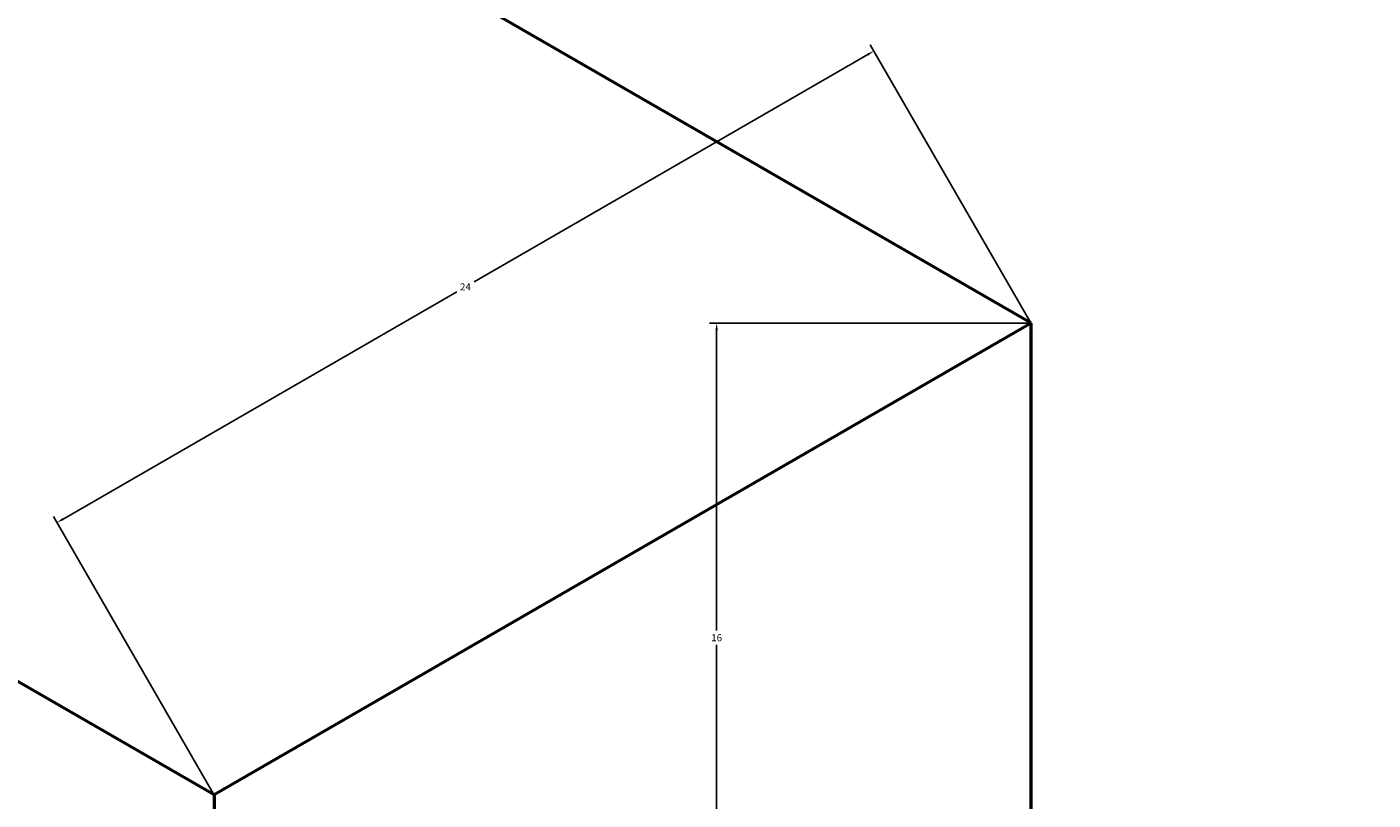
# Model space of a CAD drawing. Units: millimetres. Extents: x 2919 to 3075, y 2801 to 2951.
# Tile 11 of 14: x 3006 to 3040, y 2825 to 2844. Entities that reach past the tile are written whole.
import ezdxf

# ---------------------------------------------------------------- set-up
doc = ezdxf.new("R2010")
doc.units = ezdxf.units.MM
doc.layers.add('M-DIMS', color=2, linetype='Continuous', lineweight=18)
doc.layers.add('M-OUTL', color=7, linetype='Continuous', lineweight=50)
doc.styles.get("Standard").update_dxf_attribs({"font": 'arial.ttf'})
doc.dimstyles.get("Standard").update_dxf_attribs({"dimtxt": 0.18, "dimasz": 0.18, "dimexe": 0.18, "dimexo": 0.0625, "dimgap": 0.09, "dimtad": 0, "dimtih": 1, "dimtoh": 1, "dimdec": 4, "dimzin": 0, "dimdsep": 46, "dimtxsty": 'Standard', "dimcen": 0.09, "dimadec": 0, "dimazin": 0, "dimtfac": 1, "dimtdec": 4, "dimtofl": 0, "dimtmove": 0, "dimatfit": 3, "dimfxl": 1, "dimtolj": 1, "dimtzin": 0, "dimarcsym": 0})

# ---------------------------------------------------------------- blocks, each defined once
blk = doc.blocks.new('*D1')
at = {"layer": 'Defpoints', "color": 0, "transparency": 16777216}
for p in [(2987.323, 2944.203), (3074.337, 2944.203), (3010.912, 2808.893)]:
    blk.add_point(p, dxfattribs=at)
at = {"layer": 'M-DIMS', "color": 0, "lineweight": -2, "transparency": 16777216}
for p, q in [((2987.386, 2944.203), (3074.517, 2944.203)), ((3074.337, 2944.023), (3074.337, 2876.73)), ((3074.337, 2809.073), (3074.337, 2876.366)), ((3010.974, 2808.893), (3074.517, 2808.893))]:
    blk.add_line(p, q, dxfattribs=at)
at = {"layer": 'M-DIMS', "color": 0, "transparency": 16777216}
for points in [[(3074.307, 2944.023), (3074.367, 2944.023), (3074.337, 2944.203)], [(3074.307, 2809.073), (3074.367, 2809.073), (3074.337, 2808.893)]]:
    blk.add_solid(points, dxfattribs=at)
at = {"layer": 'M-DIMS', "color": 0, "transparency": 16777216, "insert": (3074.337, 2876.548), "char_height": 0.18, "attachment_point": 5}
blk.add_mtext('\\A1;135.3', dxfattribs=at)
blk = doc.blocks.new('*D2')
at = {"layer": 'Defpoints', "color": 0, "transparency": 16777216}
for p in [(2927.773, 2856.893), (3066.337, 2840.893), (3066.337, 2800.893)]:
    blk.add_point(p, dxfattribs=at)
at = {"layer": 'M-DIMS', "color": 0, "lineweight": -2, "transparency": 16777216}
for p, q in [((2927.773, 2856.831), (2927.773, 2800.713)), ((3066.337, 2840.831), (3066.337, 2800.713)), ((2927.953, 2800.893), (2996.6, 2800.893)), ((3066.157, 2800.893), (2997.51, 2800.893))]:
    blk.add_line(p, q, dxfattribs=at)
at = {"layer": 'M-DIMS', "color": 0, "transparency": 16777216}
for points in [[(2927.953, 2800.923), (2927.953, 2800.863), (2927.773, 2800.893)], [(3066.157, 2800.923), (3066.157, 2800.863), (3066.337, 2800.893)]]:
    blk.add_solid(points, dxfattribs=at)
at = {"layer": 'M-DIMS', "color": 0, "transparency": 16777216, "insert": (2997.055, 2800.893), "char_height": 0.18, "attachment_point": 5}
blk.add_mtext('\\A1;138.56', dxfattribs=at)
blk = doc.blocks.new('*D3')
at = {"layer": 'Defpoints', "color": 0, "transparency": 16777216}
for p in [(2927.773, 2856.893), (2923.773, 2849.965), (3010.912, 2808.893)]:
    blk.add_point(p, dxfattribs=at)
at = {"layer": 'M-DIMS', "color": 0, "lineweight": -2, "transparency": 16777216}
for p, q in [((2927.742, 2856.839), (2923.683, 2849.809)), ((2923.929, 2849.875), (2965.124, 2826.091)), ((3006.756, 2802.055), (2965.561, 2825.839)), ((3010.88, 2808.839), (3006.822, 2801.809))]:
    blk.add_line(p, q, dxfattribs=at)
at = {"layer": 'M-DIMS', "color": 0, "transparency": 16777216}
for points in [[(2923.944, 2849.901), (2923.914, 2849.849), (2923.773, 2849.965)], [(3006.771, 2802.081), (3006.741, 2802.029), (3006.912, 2801.965)]]:
    blk.add_solid(points, dxfattribs=at)
at = {"layer": 'M-DIMS', "color": 0, "transparency": 16777216, "insert": (2965.342, 2825.965), "char_height": 0.18, "attachment_point": 5}
blk.add_mtext('\\A1;96', dxfattribs=at)
blk = doc.blocks.new('*D4')
at = {"layer": 'Defpoints', "color": 0, "transparency": 16777216}
for p in [(3066.337, 2840.893), (3010.912, 2808.893), (3014.912, 2801.965)]:
    blk.add_point(p, dxfattribs=at)
at = {"layer": 'M-DIMS', "color": 0, "lineweight": -2, "transparency": 16777216}
for p, q in [((3066.368, 2840.839), (3070.427, 2833.809)), ((3070.181, 2833.875), (3042.843, 2818.092)), ((3015.068, 2802.055), (3042.405, 2817.839)), ((3010.943, 2808.839), (3015.002, 2801.809))]:
    blk.add_line(p, q, dxfattribs=at)
at = {"layer": 'M-DIMS', "color": 0, "transparency": 16777216}
for points in [[(3070.166, 2833.901), (3070.196, 2833.849), (3070.337, 2833.965)], [(3015.053, 2802.081), (3015.083, 2802.029), (3014.912, 2801.965)]]:
    blk.add_solid(points, dxfattribs=at)
at = {"layer": 'M-DIMS', "color": 0, "transparency": 16777216, "insert": (3042.624, 2817.965), "char_height": 0.18, "attachment_point": 5}
blk.add_mtext('\\A1;64', dxfattribs=at)
blk = doc.blocks.new('*D5')
at = {"layer": 'Defpoints', "color": 0, "transparency": 16777216}
for p in [(3023.696, 2836.893), (3031.696, 2836.893), (3031.696, 2820.893)]:
    blk.add_point(p, dxfattribs=at)
at = {"layer": 'M-DIMS', "color": 0, "lineweight": -2, "transparency": 16777216}
for p, q in [((3031.634, 2836.893), (3023.516, 2836.893)), ((3023.696, 2836.713), (3023.696, 2829.075)), ((3023.696, 2821.073), (3023.696, 2828.711)), ((3031.634, 2820.893), (3023.516, 2820.893))]:
    blk.add_line(p, q, dxfattribs=at)
at = {"layer": 'M-DIMS', "color": 0, "transparency": 16777216}
for points in [[(3023.666, 2836.713), (3023.726, 2836.713), (3023.696, 2836.893)], [(3023.666, 2821.073), (3023.726, 2821.073), (3023.696, 2820.893)]]:
    blk.add_solid(points, dxfattribs=at)
at = {"layer": 'M-DIMS', "color": 0, "transparency": 16777216, "insert": (3023.696, 2828.893), "char_height": 0.18, "attachment_point": 5}
blk.add_mtext('\\A1;16', dxfattribs=at)
blk = doc.blocks.new('*D6')
at = {"layer": 'Defpoints', "color": 0, "transparency": 16777216}
for p in [(3027.696, 2843.821), (3031.696, 2836.893), (3010.912, 2824.893)]:
    blk.add_point(p, dxfattribs=at)
at = {"layer": 'M-DIMS', "color": 0, "lineweight": -2, "transparency": 16777216}
for p, q in [((3031.665, 2836.947), (3027.606, 2843.977)), ((3027.54, 2843.731), (3017.524, 2837.949)), ((3007.068, 2831.911), (3017.084, 2837.694)), ((3010.88, 2824.947), (3006.822, 2831.977))]:
    blk.add_line(p, q, dxfattribs=at)
at = {"layer": 'M-DIMS', "color": 0, "transparency": 16777216}
for points in [[(3027.525, 2843.757), (3027.555, 2843.705), (3027.696, 2843.821)], [(3007.053, 2831.937), (3007.083, 2831.885), (3006.912, 2831.821)]]:
    blk.add_solid(points, dxfattribs=at)
at = {"layer": 'M-DIMS', "color": 0, "transparency": 16777216, "insert": (3017.304, 2837.821), "char_height": 0.18, "attachment_point": 5}
blk.add_mtext('\\A1;24', dxfattribs=at)

msp = doc.modelspace()

# ---------------------------------------------------------------- linework, layer by layer
at = {"layer": 'M-OUTL'}
for p, q in [((3010.9116, 2824.8932), (2941.6296, 2864.8932)), ((3031.6962, 2836.8932), (3014.3757, 2846.8932)), ((3031.6962, 2836.8932), (3010.9116, 2824.8932)), ((3031.6962, 2820.8932), (3031.6962, 2836.8932)), ((3010.9116, 2824.8932), (3010.9116, 2808.8932))]:
    msp.add_line(p, q, dxfattribs=at)

# ---------------------------------------------------------------- dimensions: what is measured, and where the dimension line sits
at = {"layer": 'M-DIMS'}
for base, p1, p2, angle, override, picture, middle in [((3074.3372, 2944.2026), (3010.9116, 2808.8932), (2987.3232, 2944.2026), 90, {"dimdec": 1, "dimlfac": 1, "dimrnd": 0, "dimzin": 0, "dimdsep": 46, "dimlunit": 2}, '*D1', (3074.3372, 2876.5479)), ((2923.7732, 2849.965), (3010.9116, 2808.8932), (2927.7732, 2856.8932), 150, {"dimdec": 0, "dimlfac": 1, "dimrnd": 0, "dimzin": 0, "dimdsep": 46, "dimlunit": 2}, '*D3', (2965.3424, 2825.965)), ((3027.6962, 2843.8214), (3010.9116, 2824.8932), (3031.6962, 2836.8932), 30, {"dimdec": 0, "dimlfac": 1, "dimrnd": 0, "dimzin": 0, "dimdsep": 46, "dimlunit": 2}, '*D6', (3017.3039, 2837.8214)), ((3014.9116, 2801.965), (3066.3372, 2840.8932), (3010.9116, 2808.8932), 210, {"dimdec": 0, "dimlfac": 1, "dimrnd": 0, "dimzin": 0, "dimdsep": 46, "dimlunit": 2}, '*D4', (3042.6244, 2817.965)), ((3023.6962, 2836.8932), (3031.6962, 2820.8932), (3031.6962, 2836.8932), 90, {"dimdec": 0, "dimlfac": 1, "dimrnd": 0, "dimzin": 0, "dimdsep": 46, "dimlunit": 2}, '*D5', (3023.6962, 2828.8932))]:
    dim = msp.add_linear_dim(base=base, p1=p1, p2=p2, angle=angle, dimstyle='Standard', override=override, dxfattribs=at)
    dim.commit()
    dim.dimension.update_dxf_attribs({"geometry": picture, "text_midpoint": middle})
dim = msp.add_linear_dim(base=(3066.3372, 2800.8932), p1=(2927.7732, 2856.8932), p2=(3066.3372, 2840.8932), dimstyle='Standard', override={"dimdec": 2, "dimlfac": 1, "dimrnd": 0, "dimzin": 0, "dimdsep": 46, "dimlunit": 2}, dxfattribs=at)
dim.commit()
dim.dimension.update_dxf_attribs({"geometry": '*D2', "text_midpoint": (2997.0552, 2800.8932)})

doc.saveas('drawing.dxf')
